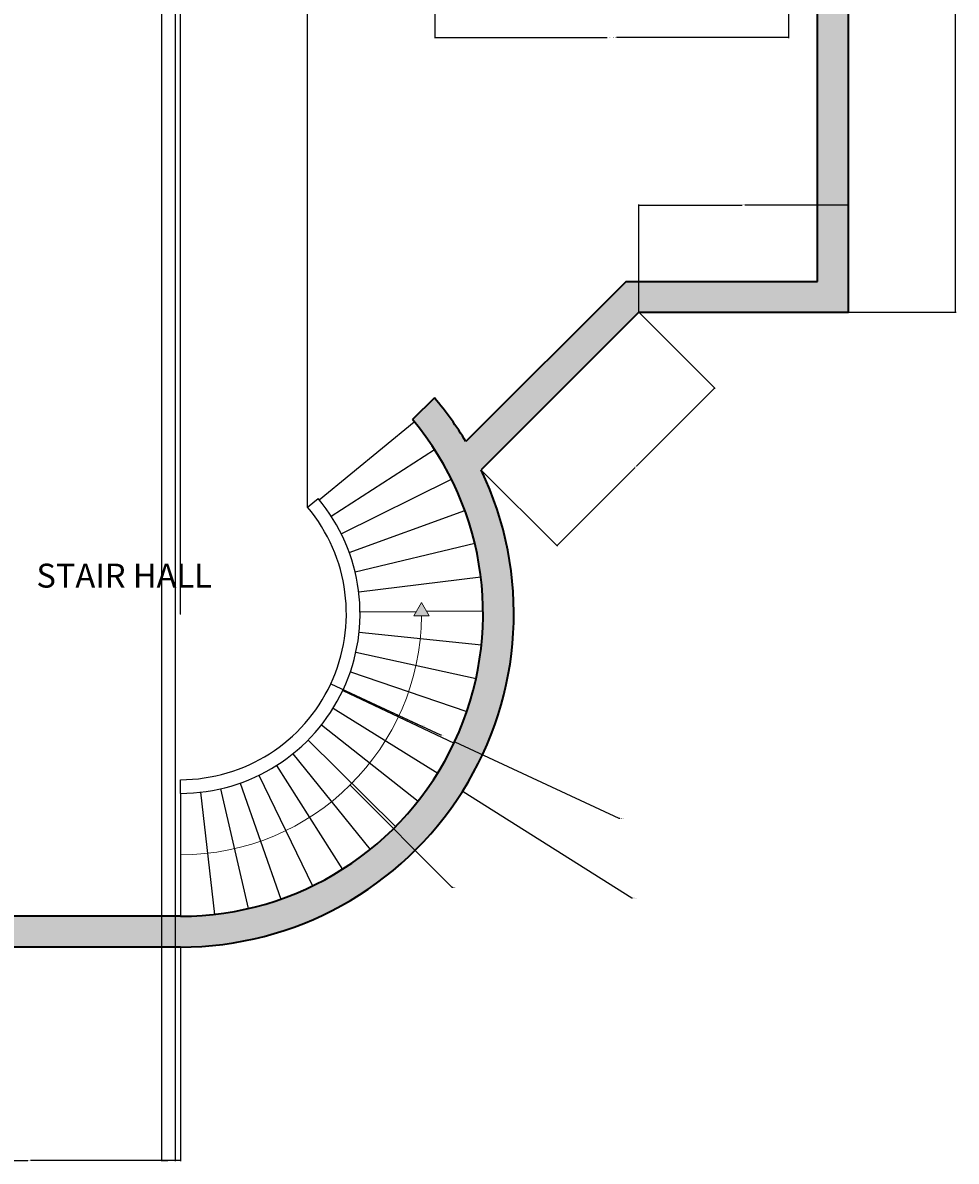
# Model space of a CAD drawing. Units: inches. Extents: x 1919 to 2461, y 2470 to 3159.
# Tile 3 of 6: x 2188 to 2461, y 2470 to 2803. Entities that reach past the tile are written whole.
import ezdxf

# ---------------------------------------------------------------- set-up
doc = ezdxf.new("R2010")
doc.units = ezdxf.units.IN
for name, color, linetype, lineweight in [('A-ANNO-DIMS', 2, 'Continuous', 18), ('A-ANNO-SYMB', 7, 'Continuous', 18), ('A-AREA-IDEN', 7, 'Continuous', 18), ('A-FLOR-STRS', 7, 'Continuous', 25), ('A-WALL', 7, 'Continuous', 35), ('A-WALL-PATT', 252, 'Continuous', 13)]:
    doc.layers.add(name, color=color, linetype=linetype, lineweight=lineweight)
doc.styles.get("Standard").update_dxf_attribs({"font": 'arial.ttf'})
doc.dimstyles.get("Standard").update_dxf_attribs({"dimtxt": 0.18, "dimasz": 0.18, "dimexe": 0.18, "dimexo": 0.0625, "dimgap": 0.09, "dimtad": 0, "dimtih": 1, "dimtoh": 1, "dimdec": 4, "dimzin": 0, "dimdsep": 46, "dimtxsty": 'Standard', "dimcen": 0.09, "dimadec": 0, "dimazin": 0, "dimtfac": 1, "dimtdec": 4, "dimtofl": 0, "dimtmove": 0, "dimatfit": 3, "dimfxl": 1, "dimtolj": 1, "dimtzin": 0, "dimarcsym": 0})

# ---------------------------------------------------------------- blocks, each defined once
blk = doc.blocks.new('*D11')
at = {"layer": 'A-ANNO-DIMS', "color": 0, "lineweight": -2, "transparency": 16777216}
for p, q in [((2308.31, 2814.5), (2308.31, 2798.86)), ((2411.85, 2814.5), (2411.85, 2798.86)), ((2308.49, 2799.04), (2358.71, 2799.04)), ((2411.67, 2799.04), (2361.45, 2799.04))]:
    blk.add_line(p, q, dxfattribs=at)
at = {"layer": 'A-ANNO-DIMS', "color": 0, "transparency": 16777216}
for points in [[(2308.49, 2799.07), (2308.49, 2799.01), (2308.31, 2799.04)], [(2411.67, 2799.07), (2411.67, 2799.01), (2411.85, 2799.04)]]:
    blk.add_solid(points, dxfattribs=at)
at = {"layer": 'Defpoints', "color": 0, "transparency": 16777216}
for p in [(2308.31, 2814.57), (2411.85, 2814.57), (2411.85, 2799.04)]:
    blk.add_point(p, dxfattribs=at)
at = {"layer": 'A-ANNO-DIMS', "color": 0, "transparency": 16777216, "insert": (2360.08, 2799.04), "char_height": 0.18, "attachment_point": 5}
blk.add_mtext('\\A1;SEATING GROUP 104', dxfattribs=at)
blk = doc.blocks.new('*D34')
at = {"layer": 'A-ANNO-DIMS', "color": 0, "lineweight": -2, "transparency": 16777216}
for p, q in [((2145.32, 2532.77), (2145.32, 2470.14)), ((2233.88, 2532.77), (2233.88, 2470.14)), ((2145.5, 2470.32), (2189.2, 2470.32)), ((2233.7, 2470.32), (2189.99, 2470.32))]:
    blk.add_line(p, q, dxfattribs=at)
at = {"layer": 'A-ANNO-DIMS', "color": 0, "transparency": 16777216}
for points in [[(2145.5, 2470.35), (2145.5, 2470.29), (2145.32, 2470.32)], [(2233.7, 2470.35), (2233.7, 2470.29), (2233.88, 2470.32)]]:
    blk.add_solid(points, dxfattribs=at)
at = {"layer": 'Defpoints', "color": 0, "transparency": 16777216}
for p in [(2145.32, 2532.83), (2233.88, 2532.83), (2233.88, 2470.32)]:
    blk.add_point(p, dxfattribs=at)
at = {"layer": 'A-ANNO-DIMS', "color": 0, "transparency": 16777216, "insert": (2189.6, 2470.32), "char_height": 0.18, "attachment_point": 5}
blk.add_mtext('\\A1;88.56', dxfattribs=at)
blk = doc.blocks.new('*D36')
at = {"layer": 'A-ANNO-DIMS', "color": 0, "lineweight": -2, "transparency": 16777216}
for p, q in [((2429.38, 3127.67), (2460.85, 3127.67)), ((2460.67, 3127.49), (2460.67, 2923.35)), ((2460.67, 2718.85), (2460.67, 2922.99)), ((2429.38, 2718.67), (2460.85, 2718.67))]:
    blk.add_line(p, q, dxfattribs=at)
at = {"layer": 'A-ANNO-DIMS', "color": 0, "transparency": 16777216}
for points in [[(2460.64, 3127.49), (2460.7, 3127.49), (2460.67, 3127.67)], [(2460.64, 2718.85), (2460.7, 2718.85), (2460.67, 2718.67)]]:
    blk.add_solid(points, dxfattribs=at)
at = {"layer": 'Defpoints', "color": 0, "transparency": 16777216}
for p in [(2429.32, 3127.67), (2460.67, 3127.67), (2429.32, 2718.67)]:
    blk.add_point(p, dxfattribs=at)
at = {"layer": 'A-ANNO-DIMS', "color": 0, "transparency": 16777216, "insert": (2460.67, 2923.17), "char_height": 0.18, "attachment_point": 5}
blk.add_mtext('\\A1;409', dxfattribs=at)
blk = doc.blocks.new('*D37')
at = {"layer": 'A-ANNO-DIMS', "color": 0, "lineweight": -2, "transparency": 16777216}
for p, q in [((2368.03, 2718.73), (2368.03, 2750.21)), ((2368.21, 2750.03), (2398.28, 2750.03)), ((2429.14, 2750.03), (2399.07, 2750.03)), ((2429.32, 2718.73), (2429.32, 2750.21))]:
    blk.add_line(p, q, dxfattribs=at)
at = {"layer": 'A-ANNO-DIMS', "color": 0, "transparency": 16777216}
for points in [[(2368.21, 2750.06), (2368.21, 2750), (2368.03, 2750.03)], [(2429.14, 2750.06), (2429.14, 2750), (2429.32, 2750.03)]]:
    blk.add_solid(points, dxfattribs=at)
at = {"layer": 'Defpoints', "color": 0, "transparency": 16777216}
for p in [(2429.32, 2750.03), (2368.03, 2718.67), (2429.32, 2718.67)]:
    blk.add_point(p, dxfattribs=at)
at = {"layer": 'A-ANNO-DIMS', "color": 0, "transparency": 16777216, "insert": (2398.67, 2750.03), "char_height": 0.18, "attachment_point": 5}
blk.add_mtext('\\A1;61.28', dxfattribs=at)
blk = doc.blocks.new('*D38')
at = {"layer": 'A-ANNO-DIMS', "color": 0, "lineweight": -2, "transparency": 16777216}
for p, q in [((2368.08, 2718.63), (2390.33, 2696.37)), ((2390.08, 2696.37), (2367.31, 2673.6)), ((2344.18, 2650.47), (2366.95, 2673.24)), ((2321.92, 2672.47), (2344.18, 2650.22))]:
    blk.add_line(p, q, dxfattribs=at)
at = {"layer": 'A-ANNO-DIMS', "color": 0, "transparency": 16777216}
for points in [[(2390.06, 2696.39), (2390.1, 2696.35), (2390.21, 2696.5)], [(2344.16, 2650.49), (2344.2, 2650.45), (2344.05, 2650.34)]]:
    blk.add_solid(points, dxfattribs=at)
at = {"layer": 'Defpoints', "color": 0, "transparency": 16777216}
for p in [(2368.03, 2718.67), (2321.88, 2672.52), (2344.05, 2650.34)]:
    blk.add_point(p, dxfattribs=at)
at = {"layer": 'A-ANNO-DIMS', "color": 0, "transparency": 16777216, "insert": (2367.13, 2673.42), "char_height": 0.18, "attachment_point": 5}
blk.add_mtext('\\A1;65.27', dxfattribs=at)
blk = doc.blocks.new('*D42')
at = {"layer": 'A-ANNO-DIMS', "color": 0, "lineweight": -2, "transparency": 16777216}
for p, q in [((2233.88, 2630.46), (2233.88, 3159.21)), ((2234.06, 3159.03), (2252.1, 3159.03)), ((2270.93, 3159.03), (2252.89, 3159.03)), ((2271.11, 2661.64), (2271.11, 3159.21))]:
    blk.add_line(p, q, dxfattribs=at)
at = {"layer": 'A-ANNO-DIMS', "color": 0, "transparency": 16777216}
for points in [[(2234.06, 3159.06), (2234.06, 3159), (2233.88, 3159.03)], [(2270.93, 3159.06), (2270.93, 3159), (2271.11, 3159.03)]]:
    blk.add_solid(points, dxfattribs=at)
at = {"layer": 'Defpoints', "color": 0, "transparency": 16777216}
for p in [(2271.11, 3159.03), (2271.11, 2661.57), (2233.88, 2630.39)]:
    blk.add_point(p, dxfattribs=at)
at = {"layer": 'A-ANNO-DIMS', "color": 0, "transparency": 16777216, "insert": (2252.49, 3159.03), "char_height": 0.18, "attachment_point": 5}
blk.add_mtext('\\A1;37.23', dxfattribs=at)
blk = doc.blocks.new('*D43')
at = {"layer": 'A-ANNO-DIMS', "color": 0, "lineweight": -2, "transparency": 16777216}
for p, q in [((2228.32, 2940.61), (2228.32, 2470.14)), ((2232.32, 2940.61), (2232.32, 2470.14)), ((2228.5, 2470.32), (2230.16, 2470.32)), ((2232.14, 2470.32), (2230.47, 2470.32))]:
    blk.add_line(p, q, dxfattribs=at)
at = {"layer": 'A-ANNO-DIMS', "color": 0, "transparency": 16777216}
for points in [[(2228.5, 2470.35), (2228.5, 2470.29), (2228.32, 2470.32)], [(2232.14, 2470.35), (2232.14, 2470.29), (2232.32, 2470.32)]]:
    blk.add_solid(points, dxfattribs=at)
at = {"layer": 'Defpoints', "color": 0, "transparency": 16777216}
for p in [(2228.32, 2940.67), (2232.32, 2940.67), (2232.32, 2470.32)]:
    blk.add_point(p, dxfattribs=at)
at = {"layer": 'A-ANNO-DIMS', "color": 0, "transparency": 16777216, "insert": (2230.32, 2470.32), "char_height": 0.18, "attachment_point": 5}
blk.add_mtext('\\A1;4', dxfattribs=at)
blk = doc.blocks.new('*D46')
at = {"layer": 'A-ANNO-DIMS', "color": 0, "lineweight": -2, "transparency": 16777216}
for p, q in [((2233.79, 2630.39), (2233.97, 2630.39)), ((2233.88, 2630.3), (2233.88, 2630.48)), ((2365.95, 2547.19), (2316.58, 2578.29)), ((2366.13, 2547.19), (2365.95, 2547.19))]:
    blk.add_line(p, q, dxfattribs=at)
at = {"layer": 'A-ANNO-DIMS', "color": 0, "transparency": 16777216}
blk.add_solid([(2316.59, 2578.32), (2316.56, 2578.27), (2316.42, 2578.39)], dxfattribs=at)
at = {"layer": 'Defpoints', "color": 0, "transparency": 16777216}
for p in [(2233.88, 2630.39), (2316.42, 2578.39)]:
    blk.add_point(p, dxfattribs=at)
at = {"layer": 'A-ANNO-DIMS', "color": 0, "transparency": 16777216, "insert": (2366.81, 2547.19), "char_height": 0.18, "attachment_point": 5}
blk.add_mtext('\\A1;4X R97.56', dxfattribs=at)
blk = doc.blocks.new('*D47')
at = {"layer": 'A-ANNO-DIMS', "color": 0, "lineweight": -2, "transparency": 16777216}
for p, q in [((2233.79, 2630.39), (2233.97, 2630.39)), ((2233.88, 2630.3), (2233.88, 2630.48)), ((2362.27, 2570.45), (2314.29, 2592.85)), ((2362.45, 2570.45), (2362.27, 2570.45))]:
    blk.add_line(p, q, dxfattribs=at)
at = {"layer": 'A-ANNO-DIMS', "color": 0, "transparency": 16777216}
blk.add_solid([(2314.3, 2592.88), (2314.27, 2592.82), (2314.12, 2592.93)], dxfattribs=at)
at = {"layer": 'Defpoints', "color": 0, "transparency": 16777216}
for p in [(2233.88, 2630.39), (2314.12, 2592.93)]:
    blk.add_point(p, dxfattribs=at)
at = {"layer": 'A-ANNO-DIMS', "color": 0, "transparency": 16777216, "insert": (2363.13, 2570.45), "char_height": 0.18, "attachment_point": 5}
blk.add_mtext('\\A1;2X R88.56', dxfattribs=at)
blk = doc.blocks.new('*D48')
at = {"layer": 'A-ANNO-DIMS', "color": 0, "lineweight": -2, "transparency": 16777216}
for p, q in [((2233.79, 2630.39), (2233.97, 2630.39)), ((2233.88, 2630.3), (2233.88, 2630.48)), ((2313.38, 2550.24), (2283.69, 2580.17)), ((2313.56, 2550.24), (2313.38, 2550.24))]:
    blk.add_line(p, q, dxfattribs=at)
at = {"layer": 'A-ANNO-DIMS', "color": 0, "transparency": 16777216}
blk.add_solid([(2283.72, 2580.19), (2283.67, 2580.15), (2283.57, 2580.3)], dxfattribs=at)
at = {"layer": 'Defpoints', "color": 0, "transparency": 16777216}
for p in [(2233.88, 2630.39), (2283.57, 2580.3)]:
    blk.add_point(p, dxfattribs=at)
at = {"layer": 'A-ANNO-DIMS', "color": 0, "transparency": 16777216, "insert": (2314.04, 2550.24), "char_height": 0.18, "attachment_point": 5}
blk.add_mtext('\\A1;R70.56', dxfattribs=at)
blk = doc.blocks.new('*D49')
at = {"layer": 'A-ANNO-DIMS', "color": 0, "lineweight": -2, "transparency": 16777216}
for p, q in [((2233.79, 2630.39), (2233.97, 2630.39)), ((2233.88, 2630.3), (2233.88, 2630.48)), ((2310.08, 2594.82), (2281.67, 2608.08)), ((2310.26, 2594.82), (2310.08, 2594.82))]:
    blk.add_line(p, q, dxfattribs=at)
at = {"layer": 'A-ANNO-DIMS', "color": 0, "transparency": 16777216}
blk.add_solid([(2281.68, 2608.11), (2281.65, 2608.05), (2281.5, 2608.16)], dxfattribs=at)
at = {"layer": 'Defpoints', "color": 0, "transparency": 16777216}
for p in [(2233.88, 2630.39), (2281.5, 2608.16)]:
    blk.add_point(p, dxfattribs=at)
at = {"layer": 'A-ANNO-DIMS', "color": 0, "transparency": 16777216, "insert": (2310.74, 2594.82), "char_height": 0.18, "attachment_point": 5}
blk.add_mtext('\\A1;R52.56', dxfattribs=at)
blk = doc.blocks.new('*D50')
at = {"layer": 'A-ANNO-DIMS', "color": 0, "lineweight": -2, "transparency": 16777216}
for p, q in [((2233.79, 2630.39), (2233.97, 2630.39)), ((2233.88, 2630.3), (2233.88, 2630.48)), ((2304.28, 2597.52), (2278.04, 2609.77)), ((2304.46, 2597.52), (2304.28, 2597.52))]:
    blk.add_line(p, q, dxfattribs=at)
at = {"layer": 'A-ANNO-DIMS', "color": 0, "transparency": 16777216}
blk.add_solid([(2278.06, 2609.8), (2278.03, 2609.75), (2277.88, 2609.85)], dxfattribs=at)
at = {"layer": 'Defpoints', "color": 0, "transparency": 16777216}
for p in [(2233.88, 2630.39), (2277.88, 2609.85)]:
    blk.add_point(p, dxfattribs=at)
at = {"layer": 'A-ANNO-DIMS', "color": 0, "transparency": 16777216, "insert": (2304.94, 2597.52), "char_height": 0.18, "attachment_point": 5}
blk.add_mtext('\\A1;R48.56', dxfattribs=at)

msp = doc.modelspace()

# ---------------------------------------------------------------- hatches: boundary and pattern name
at = {"layer": 'A-ANNO-SYMB'}
h = msp.add_hatch(color=256, dxfattribs=at)
h.dxf.hatch_style = 1
h.paths.add_polyline_path([(2304.4361, 2633.6693), (2302.2112, 2629.8157), (2306.6609, 2629.8157)])
at = {"layer": 'A-WALL-PATT'}
h = msp.add_hatch(color=256, dxfattribs=at)
h.dxf.hatch_style = 1
h.paths.add_polyline_path([(1959.315, 2931.672), (2066.315, 2931.672), (2066.315, 2940.672), (2062.315, 2940.672), (2062.315, 3005.672), (2066.315, 3005.672), (2066.315, 3009.672), (2062.315, 3009.672), (2062.315, 3118.672), (2062.315, 3127.672), (2004.315, 3127.672), (2004.315, 3072.672), (1950.315, 3072.672), (1950.315, 3059.672), (1959.315, 3059.672), (1959.315, 3063.672), (2017.315, 3063.672), (2017.315, 3067.672), (2013.315, 3067.672), (2013.315, 3118.672), (2058.315, 3118.672), (2058.315, 3067.672), (2047.315, 3067.672), (2047.315, 3063.672), (2058.315, 3063.672), (2058.315, 2940.672), (1959.315, 2940.672), (1959.315, 2952.172), (1950.315, 2952.172), (1950.315, 2901.672), (1959.315, 2901.672)])
h.paths.add_polyline_path([(2120.315, 2791.672), (2145.315, 2791.672), (2145.315, 2795.672), (2124.315, 2795.672), (2124.315, 2803.3999), (2115.315, 2803.3999), (2115.315, 2799.3999), (2067.5871, 2751.672), (1959.315, 2751.672), (1959.315, 2781.672), (1950.315, 2781.672), (1950.315, 2718.672), (1959.315, 2718.672), (1959.315, 2742.672), (2067.315, 2742.672), (2067.315, 2670.672), (2063.315, 2670.672), (2063.315, 2666.672), (2143.3108, 2666.672, 0.09553844), (2136.315, 2630.3938), (2145.315, 2630.3938, -0.2455558), (2183.315, 2703.1037), (2183.315, 2713.8315, 0.15123975), (2145.0175, 2670.672), (2071.315, 2670.672), (2071.315, 2742.672)])
h.paths.add_polyline_path([(2124.315, 2931.672), (2232.315, 2931.672), (2232.315, 2940.672), (2228.315, 2940.672), (2228.315, 2964.672), (2219.315, 2964.672), (2219.315, 2940.672), (2138.315, 2940.672), (2138.315, 3005.672), (2185.315, 3005.672), (2185.315, 3009.672), (2138.315, 3009.672), (2138.315, 3118.672), (2138.315, 3127.672), (2086.315, 3127.672), (2086.315, 3118.672), (2134.315, 3118.672), (2134.315, 3009.672), (2096.315, 3009.672), (2096.315, 3005.672), (2134.315, 3005.672), (2134.315, 2940.672), (2096.315, 2940.672), (2096.315, 2931.672), (2115.315, 2931.672), (2115.315, 2839.3999), (2124.315, 2839.3999)])
h.paths.add_polyline_path([(2429.315, 3127.672), (2384.315, 3127.672), (2384.315, 3118.672), (2420.315, 3118.672), (2420.315, 2940.672), (2268.315, 2940.672), (2268.315, 2931.672), (2420.315, 2931.672), (2420.315, 2727.672), (2364.3064, 2727.672), (2317.4188, 2680.7844, 0.0404216), (2308.2227, 2693.5694), (2301.7735, 2687.2567, -0.63673951), (2233.8773, 2541.8315), (2145.315, 2541.8315), (2145.315, 2594.3938), (2136.315, 2594.3938), (2136.315, 2510.672), (2107.815, 2510.672), (2107.815, 2501.672), (2145.315, 2501.672), (2145.315, 2532.8315), (2233.8773, 2532.8315, 0.55190633), (2321.8781, 2672.5158), (2368.0343, 2718.672), (2429.315, 2718.672)])
h.paths.add_polyline_path([(2228.315, 3118.672), (2264.315, 3118.672), (2264.315, 3127.672), (2162.315, 3127.672), (2162.315, 3118.672), (2219.315, 3118.672), (2219.315, 3009.672), (2215.315, 3009.672), (2215.315, 3005.672), (2219.315, 3005.672), (2219.315, 2994.672), (2228.315, 2994.672)], flags=0)
h.paths.add_polyline_path([(1959.315, 2666.672), (2033.315, 2666.672), (2033.315, 2670.672), (1959.315, 2670.672), (1959.315, 2694.672), (1950.315, 2694.672), (1950.315, 2501.672), (1987.815, 2501.672), (1987.815, 2510.672), (1959.315, 2510.672)])

# ---------------------------------------------------------------- linework, layer by layer
at = {"layer": 'A-ANNO-SYMB'}
msp.add_lwpolyline([(2304.4361, 2633.6693), (2302.2112, 2629.8157), (2306.6609, 2629.8157)], close=True, dxfattribs=at)
msp.add_arc((2233.8773, 2630.3938), 70.5623, 270, 359.530611, dxfattribs=at)
at = {"layer": 'A-FLOR-STRS'}
for p, q in [((2274.4992, 2663.7502), (2302.3213, 2686.5961)), ((2277.999, 2658.9608), (2308.218, 2678.5263)), ((2280.9368, 2653.8074), (2313.1679, 2669.8435)), ((2271.1076, 2661.574), (2274.1741, 2664.1423)), ((2283.2753, 2648.3559), (2317.108, 2660.6582)), ((2284.9846, 2642.6756), (2319.988, 2651.0874)), ((2286.043, 2636.8389), (2321.7713, 2641.2531)), ((2286.437, 2630.92), (2302.9442, 2631.0853)), ((2305.9108, 2631.115), (2322.4352, 2631.2805)), ((2286.1616, 2624.9945), (2321.9711, 2621.2966)), ((2285.2202, 2619.1378), (2320.3851, 2611.4285)), ((2283.625, 2613.4244), (2317.6973, 2601.802)), ((2281.3962, 2607.9271), (2313.9419, 2592.5397)), ((2278.5621, 2602.716), (2309.1669, 2583.7594)), ((2275.159, 2597.8574), (2303.4329, 2575.5732)), ((2271.2301, 2593.4132), (2296.813, 2568.0851)), ((2266.8254, 2589.4399), (2289.3916, 2561.3906)), ((2256.8186, 2583.1022), (2272.5311, 2550.7122)), ((2262.0011, 2585.9883), (2281.2631, 2555.5749)), ((2233.8773, 2577.8315), (2233.8773, 2581.8315)), ((2251.3439, 2580.8185), (2263.3069, 2546.8643)), ((2233.8773, 2577.8315), (2233.8773, 2541.8315)), ((2239.7998, 2578.1662), (2243.8561, 2542.3955)), ((2245.6468, 2579.1661), (2253.7078, 2544.0802))]:
    msp.add_line(p, q, dxfattribs=at)
for radius in [52.5623, 48.5623]:
    msp.add_arc((2233.8773, 2630.3938), radius, 270, 39.946073, dxfattribs=at)
at = {"layer": 'A-WALL'}
for p, q in [((2429.315, 2718.672), (2429.315, 3127.672)), ((2420.315, 2727.672), (2420.315, 2931.672)), ((2364.3064, 2727.672), (2317.4188, 2680.7844)), ((2364.3064, 2727.672), (2420.315, 2727.672)), ((2368.0343, 2718.672), (2321.8781, 2672.5158)), ((2368.0343, 2718.672), (2429.315, 2718.672)), ((2308.2227, 2693.5694), (2301.7735, 2687.2567)), ((2233.8773, 2541.8315), (2145.315, 2541.8315)), ((2233.8773, 2532.8315), (2145.315, 2532.8315))]:
    msp.add_line(p, q, dxfattribs=at)
for radius, start, end in [(97.5623, 31.097583, 40.35649), (88.5623, 270, 39.946073), (97.5623, 270, 25.578336)]:
    msp.add_arc((2233.8773, 2630.3938), radius, start, end, dxfattribs=at)

# ---------------------------------------------------------------- texts
at = {"layer": 'A-AREA-IDEN', "insert": (2191.7542, 2645.0614), "char_height": 7, "attachment_point": 1}
msp.add_mtext_dynamic_manual_height_columns('STAIR HALL', width=121.344683, gutter_width=12.5, heights=[0], dxfattribs=at)

# ---------------------------------------------------------------- dimensions: what is measured, and where the dimension line sits
at = {"layer": 'A-ANNO-DIMS'}
for base, p1, p2, override, picture, middle in [((2271.1076, 3159.027), (2233.8773, 2630.3938), (2271.1076, 2661.574), {"dimdec": 2, "dimlfac": 1, "dimrnd": 0, "dimzin": 0, "dimdsep": 46, "dimlunit": 2}, '*D42', (2252.4924, 3159.027)), ((2232.315, 2470.317), (2228.315, 2940.672), (2232.315, 2940.672), {"dimdec": 0, "dimlfac": 1, "dimrnd": 0, "dimzin": 0, "dimdsep": 46, "dimlunit": 2}, '*D43', (2230.315, 2470.317)), ((2429.315, 2750.027), (2368.0343, 2718.672), (2429.315, 2718.672), {"dimdec": 2, "dimlfac": 1, "dimrnd": 0, "dimzin": 0, "dimdsep": 46, "dimlunit": 2}, '*D37', (2398.6747, 2750.027)), ((2233.8773, 2470.317), (2145.315, 2532.8315), (2233.8773, 2532.8315), {"dimdec": 2, "dimlfac": 1, "dimrnd": 0, "dimzin": 0, "dimdsep": 46, "dimlunit": 2}, '*D34', (2189.5962, 2470.317))]:
    dim = msp.add_linear_dim(base=base, p1=p1, p2=p2, dimstyle='Standard', override=override, dxfattribs=at)
    dim.commit()
    dim.dimension.update_dxf_attribs({"geometry": picture, "text_midpoint": middle})
for base, p1, p2, angle, override, picture, middle in [((2460.67, 3127.672), (2429.315, 2718.672), (2429.315, 3127.672), 90, {"dimdec": 0, "dimlfac": 1, "dimrnd": 0, "dimzin": 0, "dimdsep": 46, "dimlunit": 2}, '*D36', (2460.67, 2923.172)), ((2344.0494, 2650.3445), (2368.0343, 2718.672), (2321.8781, 2672.5158), 225, {"dimdec": 2, "dimlfac": 1, "dimrnd": 0, "dimzin": 0, "dimdsep": 46, "dimlunit": 2}, '*D38', (2367.1275, 2673.4226))]:
    dim = msp.add_linear_dim(base=base, p1=p1, p2=p2, angle=angle, dimstyle='Standard', override=override, dxfattribs=at)
    dim.commit()
    dim.dimension.update_dxf_attribs({"geometry": picture, "text_midpoint": middle})
dim = msp.add_linear_dim(base=(2411.8538, 2799.0356), p1=(2308.3105, 2814.5671), p2=(2411.8538, 2814.5671), text='SEATING GROUP <>', dimstyle='Standard', override={"dimdec": 0, "dimlfac": 1, "dimrnd": 0, "dimzin": 0, "dimdsep": 46, "dimlunit": 2}, dxfattribs=at)
dim.commit()
dim.dimension.update_dxf_attribs({"geometry": '*D11', "text_midpoint": (2360.0821, 2799.0356)})
for mpoint, text, picture, middle in [((2316.4242, 2578.3899), '4X <>', '*D46', (2366.8091, 2547.1875)), ((2314.1243, 2592.9279), '2X <>', '*D47', (2363.1272, 2570.4483))]:
    dim = msp.add_radius_dim(center=(2233.8773, 2630.3938), mpoint=mpoint, text=text, dimstyle='Standard', override={"dimdec": 2, "dimlfac": 1, "dimrnd": 0, "dimzin": 0, "dimdsep": 46, "dimlunit": 2}, dxfattribs=at)
    dim.commit()
    dim.dimension.update_dxf_attribs({"geometry": picture, "text_midpoint": middle, "dimtype": 164})
for mpoint, picture, middle in [((2283.5679, 2580.2951), '*D48', (2314.042, 2550.2359)), ((2281.5045, 2608.1577), '*D49', (2310.7406, 2594.8161)), ((2277.8801, 2609.8499), '*D50', (2304.9416, 2597.5236))]:
    dim = msp.add_radius_dim(center=(2233.8773, 2630.3938), mpoint=mpoint, dimstyle='Standard', override={"dimdec": 2, "dimlfac": 1, "dimrnd": 0, "dimzin": 0, "dimdsep": 46, "dimlunit": 2}, dxfattribs=at)
    dim.commit()
    dim.dimension.update_dxf_attribs({"geometry": picture, "text_midpoint": middle, "dimtype": 164})

doc.saveas('drawing.dxf')
